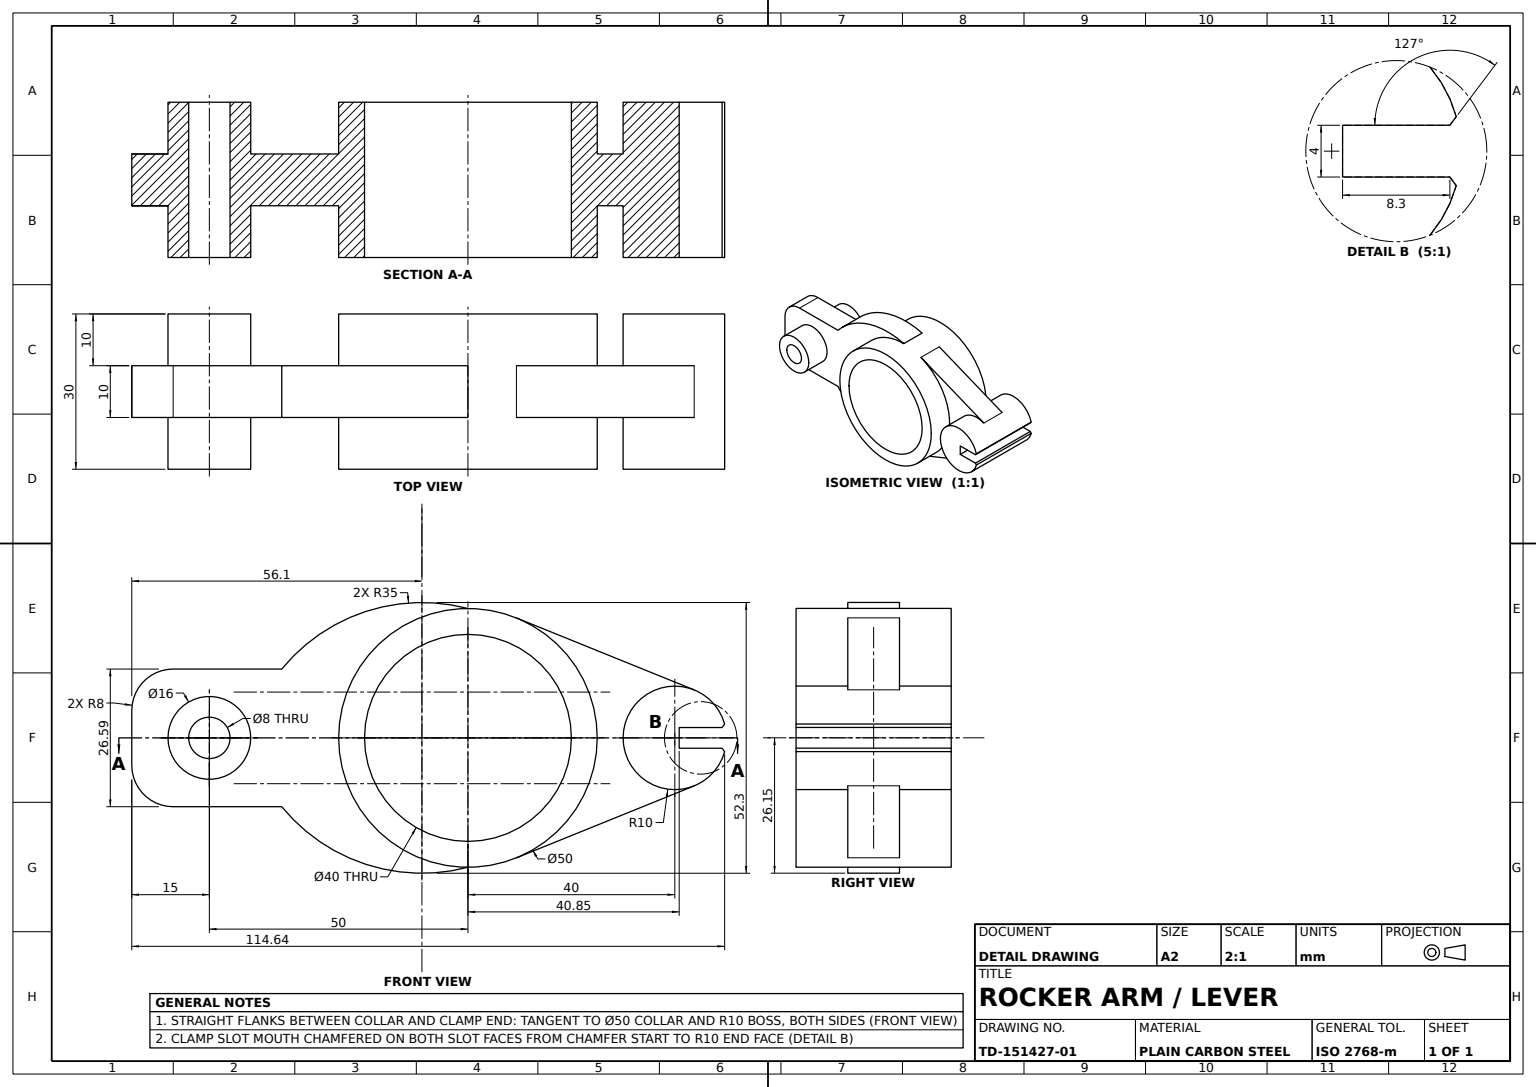
SolidWorks part; units mm, degrees
material "Plain Carbon Steel"
ref_plane "Front Plane" through (0, 0, 0) normal (0, 0, 1) x (1, 0, 0)
ref_plane "Top Plane" through (0, 0, 0) normal (0, 1, 0) x (1, 0, 0)
ref_plane "Right Plane" through (0, 0, 0) normal (1, 0, 0) x (0, 0, -1)
sketch "Collar Body Sketch" plane through (0, 0, 0) normal (0, 0, 1) x (1, 0, 0)
  circle A0 centre (0, 0) radius 25
  circle A1 centre (-50, 0) radius 8
  circle A2 centre (40, 0) radius 10
  dimension "D1" = 50
  dimension "D2" = 16
  dimension "D3" = 20
  dimension "D4" = 50
  dimension "D5" = 40
extrude "Collar Body" add sketch "Collar Body Sketch" along normal mid plane 30
sketch "Link Lugs Sketch" plane through (0, 0, 0) normal (0, 0, 1) x (1, 0, 0)
  line L0 (-65, -5.297) -> (-65, 5.297)
  line L1 (-57, 13.297) -> (-36, 13.297)
  line L2 (0, 0) -> (0, 50.177) construction
  line L3 (9.375, 23.1756) -> (43.75, 9.2702)
  line L4 (67.581, 0) -> (-83.4576, 0) construction
  line L5 (9.375, -23.1756) -> (43.75, -9.2702)
  line L6 (-57, -13.297) -> (-36, -13.297)
  line L7 (-50, 8) -> (-50, -10.4051) construction
  line L8 (-8.8982, 26.15) -> (11.9536, 26.15) construction
  line L9 (-8.8982, -26.15) -> (11.9536, -26.15) construction
  arc A0 (-36, 13.297) -> (0, 25) centre (-8.8982, -8.85) cw
  circle A1 centre (0, 0) radius 25 construction
  arc A2 (0, -25) -> (9.375, -23.1756) centre (0, 0) ccw
  circle A3 centre (40, 0) radius 10 construction
  arc A4 (43.75, -9.2702) -> (43.75, 9.2702) centre (40, 0) ccw
  arc A5 (-36, -13.297) -> (0, -25) centre (-8.8982, 8.85) ccw
  circle A6 centre (-50, 0) radius 8 construction
  arc A7 (-57, -13.297) -> (-65, -5.297) centre (-57, -5.297) cw
  arc A8 (-57, 13.297) -> (-65, 5.297) centre (-57, 5.297) ccw
  arc A9 (9.375, 23.1756) -> (0, 25) centre (0, 0) ccw
  point P24 (-65, 0)
  point P30 (-65, -13.297)
  point P33 (-65, 13.297)
  dimension "D2" = 8
  dimension "40" = 35
  dimension "D1" = 15
  dimension "D3" = 29
  dimension "D4" = 52.3
extrude "Link Lugs" add sketch "Link Lugs Sketch" along normal mid plane 10
sketch "Clamp Slot Sketch" plane through (0, 0, 15) normal (0, 0, 1) x (1, 0, 0)
  line L0 (40, 21.924) -> (40, -21.5596) construction
  line L1 (0, 0) -> (71.0848, 0) construction
  line L2 (40.8451, 2) -> (40.8451, -2)
  line L3 (40.8451, 2) -> (49.1388, 2)
  line L4 (49.1388, 2) -> (49.6388, 2.6635)
  line L5 (40.8451, -2) -> (49.1451, -2)
  line L7 (49.1451, -2) -> (49.6388, -2.6635)
  circle A0 centre (0, 0) radius 20
  circle A1 centre (-50, 0) radius 4
  circle A2 centre (-50, 0) radius 8 construction
  circle A4 centre (40, 0) radius 10 construction
  arc A5 (49.6388, -2.6635) -> (49.6388, 2.6635) centre (40, 0) ccw
  point P13 (40.8451, 0)
  dimension "D1" = 40
  dimension "D2" = 8
  dimension "D3" = 4
  dimension "D4" = 8.3
  dimension "D5" = 127
  dimension "D6" = 40.8451
  dimension "D7" = 0.5
extrude "Clamp Slot Cut" cut sketch "Clamp Slot Sketch" against normal through all
